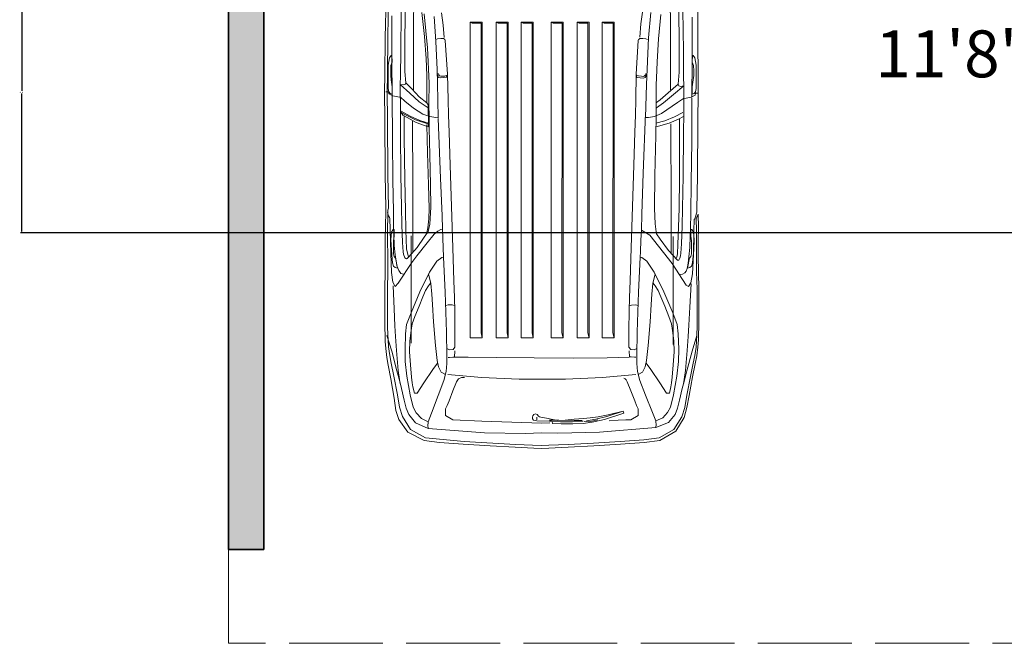
# Model space of a CAD drawing. Units: inches. Extents: x -5 to 366, y -496 to 54.
# Tile 1 of 10: x -5 to 121, y -469 to -389. Entities that reach past the tile are written whole.
import ezdxf

# ---------------------------------------------------------------- set-up
doc = ezdxf.new("R2010")
doc.units = ezdxf.units.IN
doc.header["$MEASUREMENT"] = 0
doc.linetypes.add('ACAD_ISO02W100', pattern=[15, 12, -3])
for name, color, linetype, lineweight in [('A-ANNO-DIMS', 2, 'Continuous', 18), ('A-AREA-IDEN', 7, 'Continuous', 25), ('A-FLOR-OVHD', 8, 'ACAD_ISO02W100', 18), ('A-SITE-VEHI', 8, 'Continuous', 13), ('A-WALL', 7, 'Continuous', 35), ('A-WALL-PATT', 252, 'Continuous', 13)]:
    doc.layers.add(name, color=color, linetype=linetype, lineweight=lineweight)
doc.styles.get("Standard").update_dxf_attribs({"font": 'arial.ttf'})
doc.dimstyles.get("Standard").update_dxf_attribs({"dimtxt": 0.18, "dimasz": 0.18, "dimexe": 0.18, "dimexo": 0.0625, "dimgap": 0.09, "dimtad": 0, "dimtih": 1, "dimtoh": 1, "dimdec": 0, "dimzin": 0, "dimdsep": 46, "dimlunit": 3, "dimtxsty": 'Standard', "dimcen": 0.09, "dimadec": 0, "dimazin": 0, "dimtfac": 1, "dimtdec": 0, "dimtofl": 0, "dimtmove": 0, "dimatfit": 3, "dimfxl": 1, "dimtolj": 1, "dimtzin": 0, "dimarcsym": 0})

# ---------------------------------------------------------------- blocks, each defined once
blk = doc.blocks.new('*D28')
at = {"layer": 'A-ANNO-DIMS', "color": 0, "lineweight": -2, "transparency": 16777216}
for p, q in [((165.37, -380.48), (-4.7, -380.48)), ((-4.52, -380.66), (-4.52, -398.3)), ((-4.52, -416.3), (-4.52, -398.66)), ((165.37, -416.48), (-4.7, -416.48))]:
    blk.add_line(p, q, dxfattribs=at)
at = {"layer": 'A-ANNO-DIMS', "color": 0, "transparency": 16777216}
for points in [[(-4.55, -380.66), (-4.49, -380.66), (-4.52, -380.48)], [(-4.55, -416.3), (-4.49, -416.3), (-4.52, -416.48)]]:
    blk.add_solid(points, dxfattribs=at)
at = {"layer": 'Defpoints', "color": 0, "transparency": 16777216}
for p in [(-4.52, -380.48), (165.43, -380.48), (165.43, -416.48)]:
    blk.add_point(p, dxfattribs=at)
at = {"layer": 'A-ANNO-DIMS', "color": 0, "transparency": 16777216, "insert": (-4.52, -398.48), "char_height": 0.18, "attachment_point": 5}
blk.add_mtext('\\A1;3\'-0"', dxfattribs=at)

msp = doc.modelspace()

# ---------------------------------------------------------------- hatches: boundary and pattern name
at = {"layer": 'A-WALL-PATT'}
h = msp.add_hatch(color=256, dxfattribs=at)
h.dxf.hatch_style = 1
h.paths.add_polyline_path([(324.93, 26.52), (21.93, 26.52), (21.93, -456.98), (26.43, -456.98), (26.43, -331.98), (30.93, -331.98), (30.93, -322.98), (30.93, -106.98), (110.93, -106.98), (110.93, -104.73), (110.93, -102.48), (30.93, -102.48), (30.93, 17.52), (138.93, 17.52), (141.18, 17.52), (143.43, 17.52), (183.43, 17.52), (187.93, 17.52), (315.93, 17.52), (315.93, -102.48), (315.93, -106.98), (315.93, -255.48), (171.93, -255.48), (171.93, -155.84), (167.43, -155.84), (167.43, -291.98), (171.93, -291.98), (171.93, -259.98), (315.93, -259.98), (315.93, -375.98), (297.93, -375.98), (297.93, -380.48), (315.93, -380.48), (315.93, -452.48), (315.93, -456.98), (324.93, -456.98)])
h.paths.add_polyline_path([(143.43, -18.48), (143.43, -13.98), (138.93, -13.98), (138.93, -106.98), (187.93, -106.98), (187.93, -102.48), (143.43, -102.48)], flags=17)

# ---------------------------------------------------------------- linework, layer by layer
at = {"layer": 'A-FLOR-OVHD'}
for p, q in [((21.93, -468.98), (21.93, -456.98)), ((281.67, -468.98), (21.93, -468.98))]:
    msp.add_line(p, q, dxfattribs=at)
at = {"layer": 'A-SITE-VEHI'}
for p, q in [((45.65, -382.9), (45.61, -390.12)), ((78.42, -383.06), (78.47, -390.24)), ((41.99, -391.47), (42.1, -385.84)), ((42.39, -385.7), (42.31, -391.38)), ((81.97, -386.22), (81.97, -391.88)), ((44.51, -387.97), (44.47, -392.73)), ((79.55, -387.66), (79.6, -392.61)), ((80.07, -387.94), (80.13, -393.22)), ((42.82, -388.72), (42.82, -392.56)), ((44.03, -388.16), (43.96, -393.27)), ((47, -391.35), (46.65, -388.28)), ((46.97, -388.43), (47.4, -392.78)), ((48.23, -388.8), (48.46, -391.98)), ((49.17, -388.31), (49.4, -389.89)), ((74.89, -388.23), (74.7, -389.72)), ((75.95, -388.26), (75.67, -391.5)), ((77.26, -388.52), (76.93, -391.66)), ((81.26, -388.89), (81.26, -392.72)), ((45.61, -390.12), (45.61, -395.84)), ((49.4, -389.89), (49.54, -391.48)), ((52.86, -429.91), (52.86, -389.51)), ((53.12, -389.64), (52.86, -389.51)), ((54.4, -389.51), (52.86, -389.51)), ((54.26, -389.64), (53.12, -389.64)), ((54.25, -429.26), (54.26, -389.64)), ((54.4, -389.51), (54.4, -429.91)), ((54.4, -389.51), (54.4, -429.91)), ((56.18, -429.91), (56.18, -389.51)), ((56.44, -389.64), (56.18, -389.51)), ((57.72, -389.51), (56.18, -389.51)), ((57.58, -389.64), (56.44, -389.64)), ((57.57, -429.26), (57.58, -389.64)), ((57.72, -389.51), (57.72, -429.91)), ((57.72, -389.51), (57.72, -429.91)), ((59.38, -429.91), (59.38, -389.51)), ((59.64, -389.64), (59.38, -389.51)), ((60.92, -389.51), (59.38, -389.51)), ((60.78, -389.64), (59.64, -389.64)), ((60.76, -429.26), (60.78, -389.64)), ((60.92, -389.51), (60.92, -429.91)), ((60.92, -389.51), (60.92, -429.91)), ((63.2, -429.91), (63.2, -389.51)), ((63.47, -389.64), (63.2, -389.51)), ((64.75, -389.51), (63.2, -389.51)), ((64.61, -389.64), (63.47, -389.64)), ((64.59, -429.26), (64.61, -389.64)), ((64.74, -389.51), (64.74, -429.91)), ((64.75, -389.51), (64.75, -429.91)), ((66.52, -429.91), (66.52, -389.51)), ((66.78, -389.64), (66.52, -389.51)), ((68.06, -389.51), (66.52, -389.51)), ((67.92, -389.64), (66.78, -389.64)), ((67.91, -429.26), (67.92, -389.64)), ((68.06, -389.51), (68.06, -429.91)), ((68.06, -389.51), (68.06, -429.91)), ((69.72, -429.91), (69.72, -389.51)), ((69.98, -389.64), (69.72, -389.51)), ((69.72, -389.51), (71.26, -389.51)), ((71.12, -389.64), (69.98, -389.64)), ((71.11, -429.26), (71.12, -389.64)), ((71.26, -389.51), (71.26, -429.91)), ((74.7, -389.72), (74.56, -391.43)), ((78.47, -390.24), (78.47, -395.88)), ((41.91, -396.24), (41.99, -391.47)), ((42.31, -391.38), (42.26, -396.22)), ((47.2, -394.16), (47, -391.35)), ((48.68, -391.63), (48.47, -391.75)), ((49.09, -391.59), (48.68, -391.63)), ((49.45, -391.62), (49.09, -391.59)), ((49.55, -391.67), (49.45, -391.62)), ((49.62, -391.75), (49.55, -391.67)), ((49.66, -391.84), (49.62, -391.75)), ((74.36, -391.84), (74.39, -391.75)), ((74.39, -391.75), (74.46, -391.67)), ((74.46, -391.67), (74.56, -391.62)), ((74.56, -391.62), (74.92, -391.59)), ((74.92, -391.59), (75.33, -391.63)), ((75.33, -391.63), (75.54, -391.75)), ((75.67, -391.5), (75.48, -395.51)), ((76.93, -391.66), (76.78, -394.61)), ((42.82, -392.56), (42.82, -394.29)), ((44.47, -392.73), (44.5, -395.83)), ((47.4, -392.78), (47.59, -397.31)), ((48.46, -391.98), (48.62, -395.59)), ((49.93, -396.15), (49.66, -391.84)), ((74.09, -396.15), (74.36, -391.84)), ((79.6, -392.61), (79.57, -395.9)), ((81.26, -392.72), (81.25, -394.45)), ((81.97, -391.88), (82, -396.61)), ((42.52, -394.07), (42.37, -395.03)), ((42.73, -393.76), (42.52, -394.07)), ((42.84, -393.74), (42.73, -393.76)), ((42.85, -394.64), (42.84, -393.74)), ((43.96, -393.27), (43.92, -396.4)), ((47.28, -396.34), (47.2, -394.16)), ((80.13, -393.22), (80.16, -396.53)), ((81.26, -394.64), (81.27, -393.74)), ((81.27, -393.74), (81.38, -393.76)), ((81.38, -393.76), (81.59, -394.07)), ((81.59, -394.07), (81.74, -395.03)), ((42.37, -395.03), (42.34, -396.41)), ((42.68, -395.73), (42.71, -395.08)), ((42.71, -395.08), (42.85, -394.64)), ((42.82, -394.29), (42.86, -398.92)), ((75.48, -395.51), (75.4, -397.48)), ((76.78, -394.61), (76.69, -396.69)), ((81.25, -394.45), (81.21, -399.08)), ((81.4, -395.08), (81.26, -394.64)), ((81.44, -395.73), (81.4, -395.08)), ((81.74, -395.03), (81.77, -396.41)), ((41.88, -398.41), (41.91, -396.24)), ((42.26, -396.22), (42.24, -398.41)), ((42.34, -396.41), (42.36, -397.55)), ((42.68, -396.32), (42.68, -395.73)), ((42.73, -396.9), (42.68, -396.32)), ((43.92, -396.4), (43.91, -397.47)), ((44.5, -395.83), (44.62, -397.27)), ((45.61, -395.84), (45.61, -398.16)), ((47.3, -397.22), (47.28, -396.34)), ((48.62, -395.59), (48.67, -397.31)), ((48.63, -396.13), (48.77, -396.1)), ((48.7, -396.37), (48.63, -396.13)), ((48.81, -396.58), (48.7, -396.37)), ((48.77, -396.1), (48.82, -396.25)), ((49.01, -396.65), (48.81, -396.58)), ((48.82, -396.25), (48.93, -396.39)), ((48.93, -396.39), (49.09, -396.43)), ((49.87, -396.56), (49.01, -396.65)), ((49.09, -396.43), (49.27, -396.44)), ((49.27, -396.44), (49.6, -396.43)), ((49.6, -396.43), (49.78, -396.35)), ((49.78, -396.35), (49.85, -396.45)), ((49.85, -396.45), (49.87, -396.53)), ((49.87, -396.53), (49.87, -396.56)), ((50.02, -399.43), (49.93, -396.15)), ((74.02, -399.43), (74.09, -396.15)), ((74.18, -396.29), (74.13, -396.41)), ((74.13, -396.41), (74.15, -396.54)), ((74.15, -396.54), (74.18, -396.59)), ((74.38, -396.39), (74.18, -396.29)), ((74.18, -396.59), (75.04, -396.68)), ((74.76, -396.44), (74.38, -396.39)), ((74.96, -396.46), (74.76, -396.44)), ((75.12, -396.42), (74.96, -396.46)), ((75.04, -396.68), (75.24, -396.6)), ((75.23, -396.28), (75.12, -396.42)), ((75.28, -396.13), (75.23, -396.28)), ((75.24, -396.6), (75.35, -396.4)), ((75.41, -396.15), (75.28, -396.13)), ((75.35, -396.4), (75.41, -396.15)), ((76.69, -396.69), (76.66, -397.48)), ((78.47, -395.88), (78.46, -398.16)), ((79.57, -395.9), (79.45, -397.44)), ((80.16, -396.53), (80.17, -397.68)), ((81.39, -396.9), (81.44, -396.32)), ((81.44, -396.32), (81.44, -395.73)), ((81.77, -396.41), (81.76, -397.55)), ((82, -396.61), (82.02, -398.58)), ((42.36, -397.55), (42.37, -398.02)), ((42.37, -398.02), (42.43, -398.43)), ((42.82, -397.5), (42.73, -396.9)), ((42.87, -397.77), (42.82, -397.5)), ((42.87, -398.71), (42.87, -397.77)), ((43.91, -397.47), (45.12, -398.58)), ((44.32, -397.54), (43.91, -397.47)), ((43.91, -397.47), (43.92, -401.02)), ((44.54, -397.5), (44.32, -397.54)), ((44.62, -397.27), (44.54, -397.5)), ((44.62, -397.27), (45.39, -398.04)), ((45.39, -398.04), (46.32, -399.05)), ((47.28, -399.82), (47.3, -397.22)), ((47.59, -397.31), (47.57, -399.97)), ((48.67, -397.31), (48.76, -401.75)), ((75.4, -397.48), (75.29, -401.72)), ((76.66, -397.48), (76.63, -401.53)), ((79.45, -397.44), (78.19, -398.55)), ((80.17, -397.68), (78.88, -398.77)), ((79.45, -397.44), (79.54, -397.68)), ((79.54, -397.68), (79.75, -397.74)), ((79.75, -397.74), (80.17, -397.68)), ((80.17, -397.68), (80.18, -401.07)), ((81.24, -397.77), (81.29, -397.5)), ((81.24, -398.71), (81.24, -397.77)), ((81.29, -397.5), (81.39, -396.9)), ((81.74, -398.02), (81.68, -398.43)), ((81.76, -397.55), (81.74, -398.02)), ((41.91, -402.06), (41.88, -398.41)), ((42.4, -398.42), (42.06, -398.41)), ((42.24, -398.41), (42.27, -402.06)), ((42.44, -398.69), (42.4, -398.42)), ((42.43, -398.43), (42.59, -398.63)), ((42.95, -398.95), (42.44, -398.69)), ((42.59, -398.63), (42.87, -398.71)), ((42.86, -398.92), (42.89, -404.51)), ((43.57, -399.06), (42.95, -398.95)), ((43.92, -399.13), (43.57, -399.06)), ((44.48, -399.61), (43.92, -399.13)), ((45.12, -398.58), (46.33, -399.7)), ((46.32, -399.05), (47.28, -399.82)), ((78.19, -398.55), (77.14, -399.44)), ((78.88, -398.77), (77.6, -399.82)), ((79.35, -399.81), (80.13, -399.27)), ((80.13, -399.27), (80.49, -399.22)), ((80.49, -399.22), (81.12, -399.11)), ((81.12, -399.11), (81.63, -398.85)), ((81.22, -399.18), (81.19, -404.77)), ((81.52, -398.63), (81.24, -398.71)), ((81.68, -398.43), (81.52, -398.63)), ((81.63, -398.85), (81.67, -398.58)), ((81.67, -398.58), (82, -398.58)), ((81.98, -402.23), (82.02, -398.58)), ((45.6, -400.53), (44.48, -399.61)), ((46.8, -401.3), (45.6, -400.53)), ((46.33, -399.7), (47.49, -400.47)), ((47.49, -400.11), (47.28, -399.82)), ((47.5, -402.69), (47.49, -400.11)), ((47.57, -399.97), (47.59, -401.66)), ((50.06, -401.41), (50.02, -399.43)), ((73.99, -401.41), (74.02, -399.43)), ((77.6, -399.82), (76.67, -400.46)), ((77.14, -399.44), (76.7, -399.81)), ((78.02, -400.73), (79.35, -399.81)), ((43.92, -401.02), (43.94, -403.71)), ((44.01, -400.91), (45.16, -401.56)), ((44.22, -401.42), (44.01, -401.07)), ((44.01, -401.07), (44.58, -401.39)), ((44.77, -401.73), (44.22, -401.42)), ((44.38, -401.57), (44.41, -404.26)), ((44.58, -401.39), (45.83, -402.03)), ((45.93, -402.35), (44.77, -401.73)), ((45.16, -401.56), (46.4, -402.1)), ((47.68, -401.59), (46.8, -401.3)), ((47.59, -401.66), (47.59, -401.83)), ((47.59, -401.83), (47.6, -402.32)), ((48.44, -401.72), (47.68, -401.59)), ((48.76, -401.75), (48.44, -401.72)), ((50.14, -403.57), (50.06, -401.41)), ((73.91, -403.57), (73.99, -401.41)), ((75.29, -401.15), (75, -408.85)), ((75.29, -401.72), (75.64, -401.7)), ((75.64, -401.7), (76.45, -401.58)), ((76.45, -401.58), (77.32, -401.22)), ((76.63, -401.53), (76.58, -404.02)), ((77.32, -401.22), (78.02, -400.73)), ((78.98, -401.62), (77.76, -402.14)), ((80.07, -401.06), (78.98, -401.62)), ((79.48, -401.93), (80.14, -401.57)), ((80.18, -401.07), (80.16, -403.79)), ((41.98, -409.01), (41.91, -402.06)), ((42.27, -402.06), (42.33, -409)), ((45.48, -402.16), (45.49, -410.17)), ((45.83, -402.03), (47.56, -402.58)), ((47.46, -402.9), (45.93, -402.35)), ((46.4, -402.1), (47.51, -402.44)), ((47.4, -406.25), (47.29, -402.67)), ((47.29, -402.67), (47.5, -402.69)), ((47.56, -402.58), (47.46, -402.9)), ((47.6, -402.32), (47.62, -403.06)), ((47.62, -403.06), (47.69, -406.5)), ((48.75, -401.85), (49.05, -409.49)), ((77.76, -402.14), (76.59, -402.45)), ((76.63, -402.91), (78.3, -402.44)), ((78.3, -402.44), (79.48, -401.93)), ((78.5, -402.53), (78.51, -404.98)), ((79.63, -401.88), (79.63, -404.41)), ((81.92, -409.18), (81.98, -402.23)), ((43.94, -403.71), (43.98, -409.1)), ((44.41, -404.26), (44.48, -409.63)), ((50.27, -407.81), (50.14, -403.57)), ((73.77, -407.81), (73.91, -403.57)), ((76.58, -404.02), (76.48, -409.14)), ((80.16, -403.79), (80.1, -409.23)), ((42.89, -404.51), (42.96, -409.73)), ((78.51, -404.98), (78.54, -410.44)), ((79.63, -404.41), (79.63, -409.49)), ((81.19, -404.77), (81.12, -410)), ((47.52, -410.33), (47.4, -406.25)), ((47.69, -406.5), (47.78, -410.31)), ((50.44, -413.09), (50.27, -407.81)), ((73.61, -413.09), (73.77, -407.81)), ((42.04, -413.3), (41.98, -409.01)), ((42.33, -409), (42.39, -413.29)), ((43.98, -409.1), (44.05, -413.14)), ((75, -408.85), (74.82, -414.06)), ((76.48, -409.14), (76.43, -413.34)), ((80.1, -409.23), (80.03, -413.3)), ((81.86, -413.46), (81.92, -409.18)), ((42.96, -409.73), (43.02, -413.72)), ((44.48, -409.63), (44.56, -413.67)), ((45.49, -410.17), (45.5, -415.89)), ((47.6, -413.36), (47.52, -410.33)), ((47.78, -410.31), (47.82, -413.19)), ((49.05, -409.49), (49.25, -414.3)), ((78.54, -410.44), (78.56, -416.09)), ((79.63, -409.49), (79.58, -413.36)), ((81.12, -410), (81.06, -413.99)), ((44.05, -413.14), (44.12, -415.46)), ((50.61, -418.37), (50.44, -413.09)), ((73.44, -418.37), (73.61, -413.09)), ((42.01, -415.51), (42.07, -413.84)), ((42.04, -413.48), (42.04, -413.3)), ((42.05, -413.66), (42.04, -413.48)), ((42.07, -413.84), (42.05, -413.66)), ((42.4, -414.29), (42.28, -413.88)), ((42.31, -414.41), (42.28, -415.93)), ((42.33, -413.71), (42.31, -414.41)), ((42.37, -413.43), (42.33, -413.56)), ((42.33, -413.56), (42.33, -413.71)), ((42.39, -413.29), (42.37, -413.43)), ((42.51, -414.52), (42.4, -414.29)), ((43.02, -413.72), (43.05, -415.59)), ((44.56, -413.67), (44.62, -416.11)), ((47.55, -414.69), (47.6, -413.36)), ((47.79, -413.91), (47.68, -415.37)), ((47.82, -413.19), (47.79, -413.91)), ((49.25, -414.3), (49.32, -415.97)), ((74.82, -414.06), (74.75, -416.12)), ((76.43, -413.34), (76.5, -415.32)), ((79.58, -413.36), (79.51, -415.68)), ((80.03, -413.3), (79.95, -415.62)), ((81.06, -413.99), (81.03, -415.85)), ((81.57, -414.68), (81.69, -414.42)), ((81.69, -414.42), (81.81, -413.96)), ((81.76, -414.66), (82, -414.09)), ((81.81, -413.96), (81.83, -413.81)), ((81.83, -413.81), (81.85, -413.64)), ((81.85, -413.64), (81.86, -413.46)), ((82, -414.09), (82.04, -415.73)), ((41.97, -417.4), (42.01, -415.51)), ((42.56, -414.59), (42.51, -414.52)), ((42.59, -416.07), (42.56, -414.59)), ((43.05, -415.59), (43.08, -416.65)), ((44.12, -415.46), (44.2, -417.71)), ((47.68, -415.37), (47.42, -416.48)), ((47.43, -415.83), (47.55, -414.69)), ((76.5, -415.32), (76.63, -416.32)), ((79.51, -415.68), (79.43, -417.94)), ((79.95, -415.62), (79.87, -417.88)), ((81.48, -416.23), (81.52, -414.76)), ((81.52, -414.76), (81.57, -414.68)), ((81.8, -416.16), (81.76, -414.66)), ((42.28, -415.93), (42.29, -417.55)), ((42.68, -419.08), (42.59, -416.07)), ((42.78, -416.36), (42.69, -417.32)), ((43, -416.06), (42.78, -416.36)), ((43.12, -416.04), (43, -416.06)), ((43.03, -417.49), (43.14, -416.89)), ((43.08, -416.65), (43.14, -418.07)), ((43.14, -416.89), (43.12, -416.04)), ((44.62, -416.11), (44.71, -418.5)), ((45.3, -416.85), (45.3, -430.59)), ((45.5, -415.89), (45.5, -418.95)), ((47.37, -416.43), (46.98, -417.04)), ((47.3, -416.42), (47.43, -415.83)), ((47.42, -416.48), (47.3, -416.42)), ((48.25, -416.62), (47.34, -417.75)), ((48.69, -416.27), (48.25, -416.62)), ((49.1, -416.06), (48.69, -416.27)), ((49.28, -416), (49.1, -416.06)), ((49.32, -415.97), (49.44, -419.6)), ((74.75, -416.12), (74.69, -417.42)), ((74.75, -416.12), (75.82, -416.78)), ((75.82, -416.78), (78.69, -420.41)), ((76.63, -416.32), (76.7, -416.59)), ((76.7, -416.59), (77.16, -417.29)), ((78.56, -416.09), (78.57, -419.11)), ((78.8, -416.95), (78.8, -430.77)), ((81, -416.92), (80.94, -418.33)), ((81.03, -415.85), (81, -416.92)), ((81.06, -416.89), (81.08, -416.04)), ((81.17, -417.49), (81.06, -416.89)), ((81.08, -416.04), (81.2, -416.06)), ((81.2, -416.06), (81.41, -416.36)), ((81.4, -419.25), (81.48, -416.23)), ((81.41, -416.36), (81.51, -417.32)), ((81.8, -417.74), (81.8, -416.16)), ((82.04, -415.73), (82.03, -417.55)), ((41.96, -419.33), (41.97, -417.4)), ((42.29, -417.55), (42.31, -419.33)), ((42.69, -417.32), (42.76, -418.7)), ((43.03, -418.43), (43.03, -417.49)), ((43.14, -418.07), (43.24, -419.26)), ((44.2, -417.71), (44.28, -418.91)), ((47.34, -417.75), (46.04, -419.4)), ((46.98, -417.04), (46.05, -418.35)), ((74.69, -417.42), (74.63, -418.89)), ((77.16, -417.29), (78.21, -418.74)), ((79.43, -417.94), (79.35, -419.14)), ((79.87, -417.88), (79.8, -419.08)), ((81.17, -418.43), (81.17, -417.49)), ((81.51, -417.32), (81.44, -418.7)), ((81.79, -419.5), (81.8, -417.74)), ((82.03, -417.55), (82.01, -419.44)), ((41.95, -421.36), (41.96, -419.33)), ((42.31, -419.33), (42.3, -421.36)), ((42.79, -421.55), (42.68, -419.08)), ((42.76, -418.7), (42.85, -419.83)), ((43.04, -419.16), (43.03, -418.43)), ((43.11, -419.51), (43.04, -419.16)), ((43.24, -419.26), (43.36, -420.05)), ((44.28, -418.91), (44.33, -419.18)), ((44.33, -419.18), (44.47, -419.65)), ((44.71, -418.5), (44.95, -419.56)), ((46.05, -418.35), (44.95, -419.59)), ((46.04, -419.4), (45.39, -420.25)), ((50.75, -422.61), (50.61, -418.37)), ((73.3, -422.61), (73.44, -418.37)), ((74.63, -418.89), (74.59, -419.6)), ((78.21, -418.74), (79.38, -419.96)), ((79.31, -419.38), (79.28, -419.6)), ((79.35, -419.14), (79.31, -419.38)), ((79.74, -419.39), (79.66, -419.72)), ((79.8, -419.08), (79.74, -419.39)), ((80.94, -418.33), (80.84, -419.52)), ((81.08, -419.51), (81.15, -419.16)), ((81.15, -419.16), (81.17, -418.43)), ((81.29, -421.71), (81.4, -419.25)), ((81.44, -418.7), (81.34, -419.83)), ((82.01, -419.44), (82.04, -421.44)), ((42.85, -419.83), (42.9, -420.3)), ((42.9, -420.3), (43.02, -420.71)), ((43.02, -420.71), (43.25, -420.91)), ((43.24, -419.65), (43.11, -419.51)), ((43.31, -419.68), (43.24, -419.65)), ((43.56, -420.97), (43.31, -419.68)), ((43.36, -420.05), (43.47, -420.64)), ((43.47, -420.64), (43.59, -420.98)), ((45.39, -420.25), (43.64, -422.91)), ((44.47, -419.65), (44.7, -419.79)), ((44.7, -419.79), (44.78, -419.73)), ((44.78, -419.73), (44.86, -419.66)), ((44.86, -419.66), (44.95, -419.59)), ((48.58, -420.1), (47.63, -421.48)), ((49.21, -419.64), (48.58, -420.1)), ((49.44, -419.6), (49.21, -419.64)), ((49.44, -419.6), (49.65, -424.06)), ((74.59, -419.6), (74.38, -424.06)), ((74.59, -419.6), (74.82, -419.64)), ((74.82, -419.64), (75.46, -420.1)), ((75.46, -420.1), (76.4, -421.48)), ((78.69, -420.41), (80.46, -423.17)), ((79.28, -419.6), (79.18, -419.77)), ((79.38, -419.96), (79.44, -419.98)), ((79.44, -419.98), (79.49, -419.98)), ((79.49, -419.98), (79.54, -419.95)), ((79.66, -419.72), (79.54, -419.95)), ((80.72, -420.35), (80.59, -421.01)), ((80.63, -420.97), (80.89, -419.68)), ((80.84, -419.52), (80.72, -420.35)), ((80.89, -419.68), (80.95, -419.65)), ((80.95, -419.65), (81.08, -419.51)), ((81.18, -420.71), (80.95, -420.91)), ((81.3, -420.3), (81.18, -420.71)), ((81.34, -419.83), (81.3, -420.3)), ((81.82, -421.46), (81.79, -419.5)), ((41.93, -423.7), (41.95, -421.36)), ((42.3, -421.36), (42.28, -423.7)), ((42.95, -422.79), (42.79, -421.55)), ((43.25, -420.91), (43.56, -420.97)), ((43.59, -420.98), (43.73, -421.29)), ((43.73, -421.29), (43.96, -421.65)), ((43.96, -421.65), (44.32, -421.74)), ((47.63, -421.48), (46.42, -424.02)), ((47.52, -421.71), (47.81, -422.94)), ((76.52, -421.71), (76.23, -422.94)), ((76.4, -421.48), (77.61, -424.02)), ((80.03, -421.75), (79.63, -421.78)), ((80.31, -421.59), (80.03, -421.75)), ((80.47, -421.38), (80.31, -421.59)), ((80.59, -421.01), (80.47, -421.38)), ((80.95, -420.91), (80.63, -420.97)), ((81.08, -422.86), (81.29, -421.71)), ((81.87, -423.66), (81.82, -421.46)), ((82.04, -421.44), (82.09, -423.73)), ((43.23, -423.33), (42.95, -422.79)), ((43.64, -422.91), (43.23, -423.33)), ((47.5, -423.25), (47.15, -423.83)), ((47.79, -422.91), (47.5, -423.25)), ((47.81, -422.94), (47.96, -424.33)), ((50.83, -424.75), (50.75, -422.61)), ((73.22, -424.75), (73.3, -422.61)), ((76.23, -422.94), (76.08, -424.33)), ((76.25, -422.91), (76.53, -423.25)), ((76.53, -423.25), (76.89, -423.83)), ((80.46, -423.17), (80.77, -423.34)), ((80.77, -423.34), (81.08, -422.86)), ((81.11, -423), (80.97, -425.98)), ((41.92, -426.37), (41.93, -423.7)), ((42.28, -423.7), (42.27, -426.37)), ((42.99, -423.26), (43.11, -426.17)), ((46.42, -424.02), (45.28, -426.72)), ((47.15, -423.83), (46.79, -424.64)), ((47.96, -424.33), (48.02, -425.64)), ((49.65, -424.06), (49.81, -429.18)), ((74.38, -424.06), (74.23, -429.18)), ((76.08, -424.33), (76.02, -425.64)), ((76.89, -423.83), (77.25, -424.64)), ((77.61, -424.02), (78.76, -426.72)), ((81.89, -426.25), (81.87, -423.66)), ((82.09, -423.73), (82.12, -426.37)), ((46.79, -424.64), (46.31, -425.83)), ((48.02, -425.64), (48.16, -427.85)), ((49.74, -425.75), (50.02, -425.66)), ((50.02, -425.66), (50.54, -425.67)), ((50.54, -425.67), (50.82, -425.77)), ((50.87, -426.48), (50.83, -424.75)), ((73.18, -426.48), (73.22, -424.75)), ((73.5, -425.7), (73.23, -425.8)), ((74.02, -425.69), (73.5, -425.7)), ((74.3, -425.78), (74.02, -425.69)), ((76.02, -425.64), (75.88, -427.85)), ((77.25, -424.64), (77.73, -425.83)), ((41.94, -428.52), (41.92, -426.37)), ((42.27, -426.37), (42.29, -428.47)), ((43.11, -426.17), (43.22, -428.37)), ((45.28, -426.72), (44.71, -428.21)), ((46.31, -425.83), (45.76, -427.18)), ((50.89, -428.89), (50.87, -426.48)), ((73.16, -428.89), (73.18, -426.48)), ((77.73, -425.83), (78.27, -427.18)), ((78.76, -426.72), (79.33, -428.21)), ((80.97, -425.98), (80.83, -428.3)), ((81.87, -428.41), (81.89, -426.25)), ((82.12, -426.37), (82.1, -428.47)), ((44.71, -428.21), (44.59, -429.39)), ((45.44, -428.1), (45.29, -428.96)), ((45.76, -427.18), (45.44, -428.1)), ((48.16, -427.85), (48.41, -430.86)), ((75.88, -427.85), (75.62, -430.86)), ((78.27, -427.18), (78.59, -428.1)), ((78.59, -428.1), (78.74, -428.96)), ((79.33, -428.21), (79.44, -429.39)), ((80.83, -428.3), (80.75, -429.71)), ((41.97, -429.67), (41.94, -428.52)), ((42.29, -428.47), (42.33, -429.53)), ((42.33, -429.53), (42.35, -430.17)), ((43.22, -428.37), (43.29, -429.71)), ((44.59, -429.39), (44.51, -431.33)), ((45.29, -428.96), (45.14, -430.29)), ((49.81, -429.18), (49.86, -432.17)), ((50.89, -431.11), (50.89, -428.89)), ((54.4, -429.91), (54.25, -429.26)), ((57.72, -429.91), (57.57, -429.26)), ((60.92, -429.91), (60.76, -429.26)), ((64.74, -429.91), (64.59, -429.26)), ((68.06, -429.91), (67.91, -429.26)), ((71.26, -429.91), (71.11, -429.26)), ((73.16, -431.11), (73.16, -428.89)), ((74.23, -429.18), (74.17, -432.17)), ((78.74, -428.96), (78.89, -430.29)), ((79.44, -429.39), (79.53, -431.33)), ((81.84, -429.57), (81.87, -428.41)), ((82.06, -429.53), (82.04, -430.17)), ((82.1, -428.47), (82.06, -429.53)), ((41.98, -430.37), (41.97, -429.67)), ((42.04, -431.28), (41.98, -430.37)), ((42.17, -429.6), (42.81, -431.62)), ((42.35, -430.17), (42.41, -431.05)), ((43.29, -429.71), (43.41, -431.52)), ((45.14, -430.29), (45.1, -431.71)), ((54.4, -429.91), (52.86, -429.91)), ((57.72, -429.91), (56.18, -429.91)), ((60.92, -429.91), (59.38, -429.91)), ((64.75, -429.91), (63.2, -429.91)), ((68.06, -429.91), (66.52, -429.91)), ((71.26, -429.91), (69.72, -429.91)), ((78.89, -430.29), (78.94, -431.71)), ((80.75, -429.71), (80.62, -431.52)), ((81.86, -429.6), (81.23, -431.62)), ((81.75, -431.11), (81.82, -430.27)), ((81.82, -430.27), (81.84, -429.57)), ((82.04, -430.17), (81.98, -431.08)), ((42.19, -432.41), (42.04, -431.28)), ((42.41, -431.05), (42.55, -432.15)), ((42.81, -431.62), (43.47, -434.1)), ((43.41, -431.52), (43.65, -434.09)), ((44.51, -431.33), (44.52, -432.94)), ((45.1, -431.71), (45.2, -433.34)), ((48.41, -430.86), (48.63, -432.79)), ((49.88, -431.26), (50.21, -431.45)), ((50.21, -431.45), (50.66, -431.39)), ((50.66, -431.39), (50.89, -431.11)), ((50.89, -431.58), (50.86, -432.37)), ((73.38, -431.39), (73.16, -431.11)), ((73.18, -431.55), (73.21, -432.33)), ((73.84, -431.45), (73.38, -431.39)), ((74.17, -431.26), (73.84, -431.45)), ((75.62, -430.86), (75.4, -432.79)), ((78.94, -431.71), (78.83, -433.34)), ((79.53, -431.33), (79.52, -432.94)), ((80.62, -431.52), (80.39, -434.09)), ((81.23, -431.62), (80.56, -434.1)), ((81.57, -432.17), (81.75, -431.11)), ((81.98, -431.08), (81.84, -432.21)), ((42.37, -433.41), (42.19, -432.41)), ((42.55, -432.15), (42.73, -433.13)), ((42.73, -433.13), (43.08, -434.82)), ((44.52, -432.94), (44.76, -434.79)), ((45.2, -433.34), (45.36, -434.95)), ((48.09, -433.97), (48.67, -433.14)), ((48.63, -432.79), (48.81, -433.59)), ((49.87, -433.17), (49.78, -434.21)), ((49.86, -432.17), (49.87, -433.17)), ((50.22, -432.4), (50.02, -432.41)), ((50.64, -432.38), (50.22, -432.4)), ((50.86, -432.37), (50.64, -432.38)), ((52.57, -432.37), (50.86, -432.37)), ((56.26, -432.42), (52.57, -432.37)), ((61.04, -432.47), (56.26, -432.42)), ((66.05, -432.49), (61.04, -432.47)), ((70.38, -432.47), (66.05, -432.49)), ((73.17, -432.37), (70.38, -432.47)), ((73.21, -432.33), (73.43, -432.34)), ((73.43, -432.34), (73.85, -432.36)), ((73.85, -432.36), (74.05, -432.37)), ((74.17, -432.17), (74.17, -433.17)), ((74.17, -433.17), (74.25, -434.21)), ((75.4, -432.79), (75.23, -433.59)), ((75.95, -433.97), (75.36, -433.14)), ((78.83, -433.34), (78.68, -434.95)), ((79.52, -432.94), (79.27, -434.79)), ((81.03, -434.83), (81.37, -433.13)), ((81.65, -433.22), (81.31, -434.89)), ((81.37, -433.13), (81.57, -432.17)), ((81.84, -432.21), (81.65, -433.22)), ((42.7, -435.14), (42.37, -433.41)), ((43.47, -434.1), (43.83, -435.48)), ((43.65, -434.09), (43.9, -435.79)), ((46.92, -435.66), (48.09, -433.97)), ((48.81, -433.59), (49.12, -434.28)), ((49.12, -434.28), (49.71, -434.6)), ((49.78, -434.21), (49.48, -435.37)), ((54.31, -434.96), (49.98, -434.6)), ((74.06, -434.6), (69.77, -434.96)), ((74.25, -434.21), (74.56, -435.37)), ((74.91, -434.28), (74.33, -434.6)), ((75.23, -433.59), (74.91, -434.28)), ((77.11, -435.66), (75.95, -433.97)), ((80.39, -434.09), (80.13, -435.79)), ((80.56, -434.1), (80.21, -435.48)), ((43.11, -437.61), (42.7, -435.14)), ((43.08, -434.82), (43.54, -437.21)), ((43.83, -435.48), (44.05, -436.4)), ((44.76, -434.79), (45.19, -437.21)), ((45.36, -434.95), (45.44, -435.67)), ((45.44, -435.67), (45.51, -436.18)), ((46.06, -436.98), (46.92, -435.66)), ((49.48, -435.37), (48.76, -437.28)), ((50.63, -436.67), (51.1, -435.52)), ((51.1, -435.52), (51.37, -435.14)), ((51.37, -435.14), (51.72, -434.98)), ((51.72, -434.98), (52.11, -434.98)), ((59.1, -435.17), (54.31, -434.96)), ((62.1, -435.17), (59.1, -435.17)), ((65.05, -435.17), (62.1, -435.17)), ((69.77, -434.96), (65.05, -435.17)), ((72.49, -435.04), (72.66, -435.14)), ((72.66, -435.14), (72.81, -435.29)), ((72.81, -435.29), (72.94, -435.52)), ((72.94, -435.52), (73.4, -436.67)), ((74.56, -435.37), (75.29, -437.25)), ((77.98, -436.98), (77.11, -435.66)), ((78.59, -435.67), (78.53, -436.18)), ((78.68, -434.95), (78.59, -435.67)), ((79.27, -434.79), (78.85, -437.21)), ((80.21, -435.48), (79.98, -436.4)), ((80.56, -437.25), (81.03, -434.83)), ((81.31, -434.89), (80.85, -437.27)), ((44.05, -436.4), (44.42, -437.88)), ((45.51, -436.18), (45.71, -436.97)), ((45.71, -436.97), (46.06, -436.98)), ((50.14, -437.95), (50.63, -436.67)), ((73.4, -436.67), (73.9, -437.95)), ((78.33, -436.97), (77.98, -436.98)), ((78.53, -436.18), (78.33, -436.97)), ((79.98, -436.4), (79.62, -437.88)), ((43.35, -439.21), (43.11, -437.61)), ((43.54, -437.21), (43.81, -438.77)), ((44.42, -437.88), (44.67, -438.91)), ((45.19, -437.21), (45.56, -438.75)), ((48.76, -437.28), (47.9, -439.54)), ((49.9, -438.56), (50.14, -437.95)), ((73.9, -437.95), (74.13, -438.56)), ((75.29, -437.25), (76.18, -439.45)), ((78.85, -437.21), (78.48, -438.75)), ((79.62, -437.88), (79.36, -438.91)), ((80.29, -438.83), (80.56, -437.25)), ((80.85, -437.27), (80.58, -438.81)), ((43.73, -440.36), (43.35, -439.21)), ((43.81, -438.77), (44.17, -439.96)), ((44.67, -438.91), (44.99, -439.72)), ((45.56, -438.75), (45.95, -439.48)), ((45.95, -439.48), (46.6, -440.21)), ((47.9, -439.54), (47.48, -440.63)), ((49.68, -439.85), (49.71, -439)), ((49.71, -439), (49.9, -438.56)), ((61, -439.7), (61.19, -439.63)), ((61.19, -439.63), (61.4, -439.72)), ((70.05, -440.33), (72.52, -439.54)), ((72.44, -439.29), (70.32, -439.97)), ((72.44, -439.29), (70.49, -439.77)), ((72.52, -439.54), (72.44, -439.29)), ((74.13, -438.56), (74.33, -439)), ((74.33, -439), (74.36, -439.85)), ((76.18, -439.45), (76.61, -440.51)), ((78.1, -439.45), (77.48, -440.12)), ((78.48, -438.75), (78.1, -439.45)), ((79.36, -438.91), (79.06, -439.69)), ((79.94, -440), (80.29, -438.83)), ((80.58, -438.81), (80.22, -440.07)), ((44.86, -441.95), (43.73, -440.36)), ((44.17, -439.96), (45.22, -441.61)), ((44.99, -439.72), (45.85, -440.79)), ((45.85, -440.79), (47.48, -441.48)), ((46.6, -440.21), (47.48, -440.63)), ((47.46, -440.77), (47.45, -441.09)), ((47.48, -440.63), (47.46, -440.77)), ((50.63, -440.37), (49.68, -439.85)), ((54.35, -440.54), (50.63, -440.37)), ((59.45, -440.73), (54.35, -440.54)), ((62.02, -440.83), (59.45, -440.73)), ((60.82, -440.03), (60.86, -439.88)), ((60.83, -440.25), (60.82, -440.03)), ((60.93, -440.45), (60.83, -440.25)), ((60.86, -439.88), (61, -439.7)), ((61.39, -440.52), (60.93, -440.45)), ((61.36, -440.39), (61.38, -440.05)), ((63, -440.56), (61.39, -440.52)), ((61.4, -439.72), (61.59, -439.9)), ((61.59, -439.9), (61.73, -440)), ((61.9, -440.03), (61.73, -440)), ((62.59, -440.16), (61.9, -440.03)), ((63.04, -440.79), (62.02, -440.83)), ((64.03, -440.46), (62.59, -440.16)), ((64.19, -440.45), (62.99, -440.45)), ((63.23, -440.56), (63, -440.56)), ((64.42, -440.66), (63.33, -440.62)), ((63.33, -440.62), (63.4, -440.88)), ((63.4, -440.88), (64.5, -440.91)), ((66.14, -440.46), (64.19, -440.45)), ((65.92, -440.66), (64.42, -440.66)), ((66.17, -440.32), (65, -440.45)), ((67.25, -440.58), (65.92, -440.66)), ((66, -440.91), (67.32, -440.84)), ((67.17, -440.46), (66.14, -440.46)), ((67.33, -440.21), (66.17, -440.32)), ((67.26, -440.58), (67.25, -440.58)), ((67.28, -440.58), (67.26, -440.58)), ((67.29, -440.58), (67.28, -440.58)), ((67.32, -440.84), (68.46, -440.69)), ((68.2, -440.13), (67.33, -440.21)), ((68.01, -440.63), (67.44, -440.59)), ((68.91, -440.31), (67.74, -440.51)), ((68.18, -440.6), (68.01, -440.63)), ((68.62, -440.51), (68.18, -440.6)), ((69.22, -440), (68.2, -440.13)), ((68.46, -440.69), (70.05, -440.33)), ((69.18, -440.38), (68.62, -440.51)), ((70.32, -439.97), (68.91, -440.31)), ((70.49, -439.77), (69.22, -440)), ((71.8, -440.45), (70.61, -440.5)), ((72.75, -440.4), (71.8, -440.45)), ((73.4, -440.37), (72.75, -440.4)), ((74.36, -439.85), (73.4, -440.37)), ((77.48, -440.12), (76.61, -440.51)), ((76.61, -440.51), (76.62, -440.65)), ((78.22, -440.71), (76.61, -441.36)), ((76.62, -440.65), (76.64, -440.97)), ((79.06, -439.69), (78.22, -440.71)), ((78.91, -441.62), (79.94, -440)), ((80.22, -440.07), (79.15, -441.85)), ((46.95, -443.04), (44.86, -441.95)), ((45.22, -441.61), (47.11, -442.71)), ((47.45, -441.09), (47.48, -441.48)), ((54.68, -442.07), (47.48, -441.48)), ((59.94, -442.13), (54.68, -442.07)), ((61.98, -442.06), (59.94, -442.13)), ((64.05, -442.1), (61.98, -442.06)), ((69.38, -441.98), (64.05, -442.1)), ((64.5, -440.91), (66, -440.91)), ((76.61, -441.36), (69.38, -441.98)), ((76.64, -440.97), (76.61, -441.36)), ((77.02, -442.69), (78.91, -441.62)), ((79.15, -441.85), (77.09, -443.04)), ((48.93, -443.29), (46.95, -443.04)), ((47.11, -442.71), (52.06, -443.18)), ((51.95, -443.52), (48.93, -443.29)), ((52.06, -443.18), (58.65, -443.54)), ((65.37, -443.54), (68.63, -443.38)), ((68.63, -443.38), (72.05, -443.17)), ((72.05, -443.17), (75.05, -442.94)), ((75.11, -443.29), (72.09, -443.52)), ((75.05, -442.94), (77.02, -442.69)), ((77.09, -443.04), (75.11, -443.29)), ((55.39, -443.73), (51.95, -443.52)), ((58.61, -443.9), (55.39, -443.73)), ((61, -444), (58.61, -443.9)), ((58.65, -443.54), (61.95, -443.69)), ((61.93, -444.04), (61, -444)), ((62.91, -444), (61.93, -444.04)), ((61.95, -443.69), (62.92, -443.65)), ((65.38, -443.9), (62.91, -444)), ((62.92, -443.65), (65.37, -443.54)), ((68.65, -443.73), (65.38, -443.9)), ((72.09, -443.52), (68.65, -443.73))]:
    msp.add_line(p, q, dxfattribs=at)
at = {"layer": 'A-WALL'}
for p, q in [((21.93, 26.52), (21.93, -456.98)), ((26.43, -331.98), (26.43, -456.98)), ((26.43, -456.98), (21.93, -456.98))]:
    msp.add_line(p, q, dxfattribs=at)

# ---------------------------------------------------------------- texts
at = {"layer": 'A-AREA-IDEN', "insert": (104.68, -380.57), "char_height": 6, "attachment_point": 1}
msp.add_mtext('PARKING\\P11\'8"X10\'4\'\'', dxfattribs=at)

# ---------------------------------------------------------------- dimensions: what is measured, and where the dimension line sits
at = {"layer": 'A-ANNO-DIMS'}
dim = msp.add_linear_dim(base=(-4.52, -380.48), p1=(165.43, -416.48), p2=(165.43, -380.48), angle=90, dimstyle='Standard', override={"dimdec": 1, "dimlfac": 1, "dimrnd": 0, "dimzin": 1, "dimdsep": 46, "dimlunit": 4, "dimfrac": 2}, dxfattribs=at)
dim.commit()
dim.dimension.update_dxf_attribs({"geometry": '*D28', "text_midpoint": (-4.52, -398.48)})

doc.saveas('drawing.dxf')
